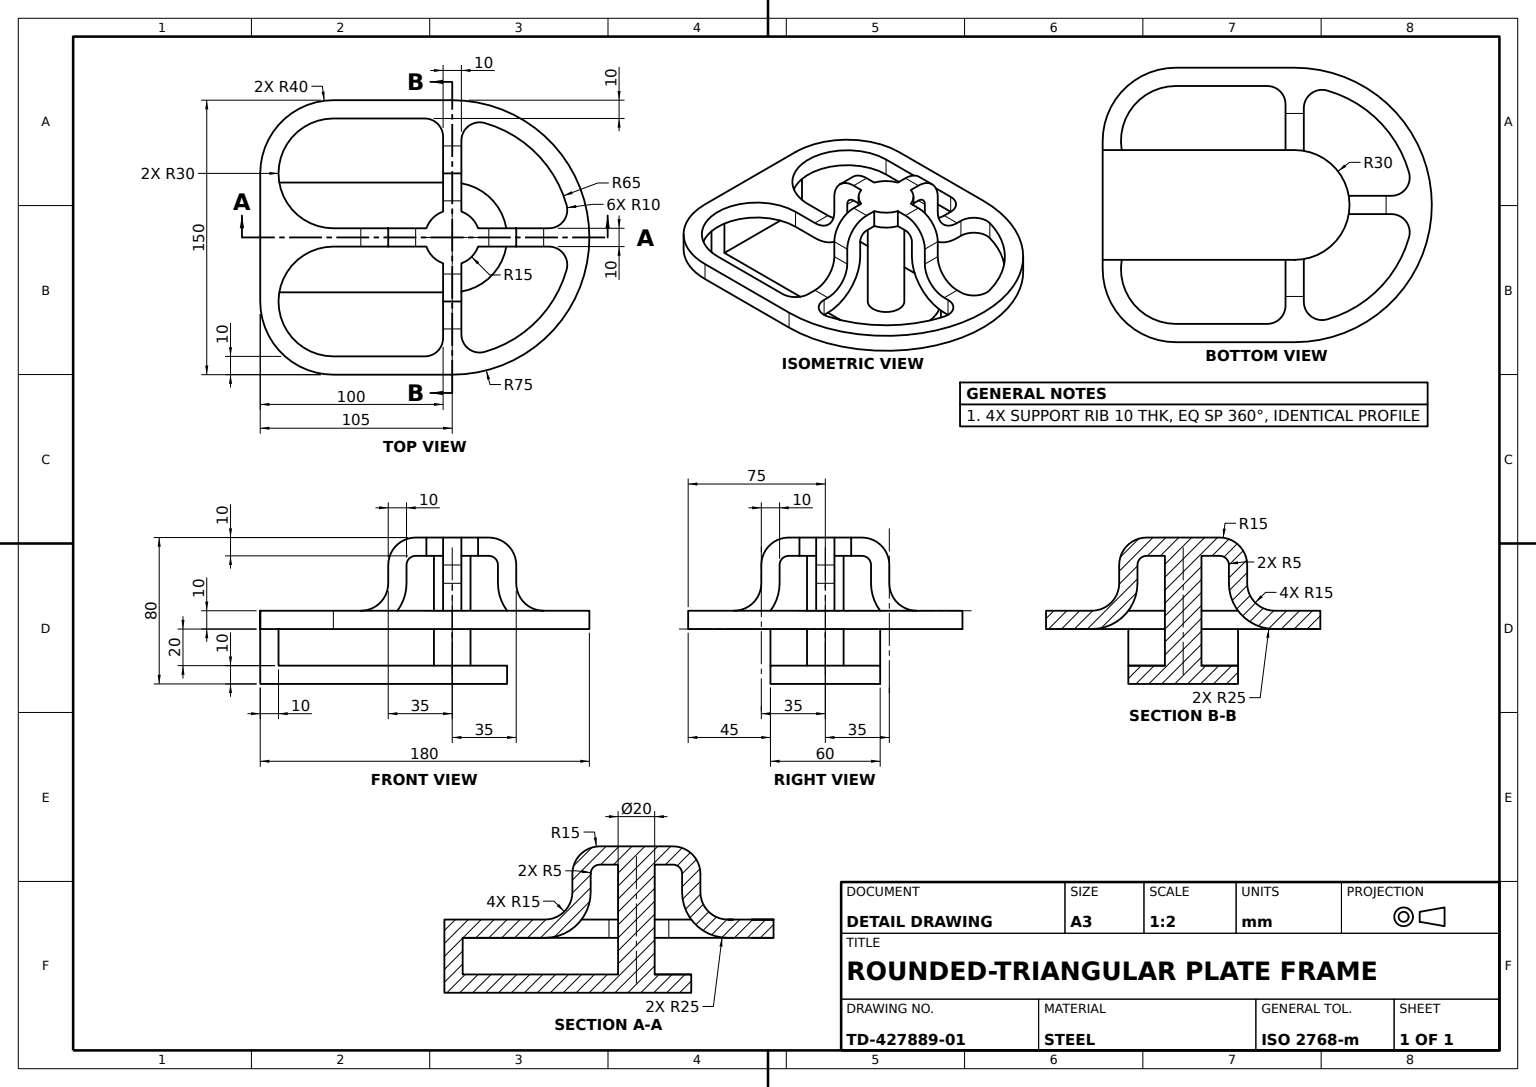
from build123d import *

# Parameters (mm, degrees)
CENTRAL_POST_SKETCH_R       = 10
CENTRAL_POST_20_DEPTH       = 40
MOUNTING_PLATE_DEPTH        = 10
RECTANGULAR_PAD_60X30_DEPTH = 10
SIDE_WALL_SKETCH_W          = 10
SIDE_WALL_SKETCH_H          = 20
SIDE_WALL_DEPTH             = 30
HUB_SKETCH_R                = 15
HUB_30_DEPTH                = 10
PLATE_CUTOUTS_SKETCH_R      = 10
PLATE_CUTOUTS_DEPTH         = 10
SUPPORT_RIB_DEPTH           = 5
RIB_PATTERN_4X_COUNT        = 4


with BuildPart() as part:
    # Central Post Sketch → Central Post Ø20 (new, symmetric)
    with BuildSketch(Plane(origin=(0, 0, 0), x_dir=(1, 0, 0), z_dir=(0, 1, 0))):
        with Locations(Location((0, 0, 0), (0, 0, 270))):
            Circle(CENTRAL_POST_SKETCH_R)
    extrude(amount=CENTRAL_POST_20_DEPTH, both=True)

    # Plate Outline Sketch → Mounting Plate (add)
    with BuildSketch(Plane(origin=(0, 0, 0), x_dir=(1, 0, 0), z_dir=(0, 1, 0))):
        with BuildLine():
            Line((-65, 75), (0, 75))
            ThreePointArc((0, 75), (75, 0), (0, -75))
            Line((0, -75), (-65, -75))
            ThreePointArc((-65, -75), (-93.284271247, -63.284271247), (-105, -35))
            Line((-105, -35), (-105, 35))
            ThreePointArc((-105, 35), (-93.284271247, 63.284271247), (-65, 75))
        make_face()
    extrude(amount=-MOUNTING_PLATE_DEPTH)

    # Pad Sketch → Rectangular Pad 60x30 (add)
    with BuildSketch(Plane.XZ.offset(40)):
        with BuildLine():
            Line((-105, 30), (0, 30))
            ThreePointArc((0, 30), (30, 0), (0, -30))
            Line((0, -30), (-105, -30))
            Line((-105, -30), (-105, 30))
        make_face()
    extrude(amount=-RECTANGULAR_PAD_60X30_DEPTH)

    # Side Wall Sketch → Side Wall (add, symmetric)
    with BuildSketch(Plane.XY):
        with Locations((-100, -20)):
            Rectangle(SIDE_WALL_SKETCH_W, SIDE_WALL_SKETCH_H)
    extrude(amount=SIDE_WALL_DEPTH, both=True)

    # Hub Sketch → Hub Ø30 (add)
    with BuildSketch(Plane(origin=(0, 40, 0), x_dir=(1, 0, 0), z_dir=(0, 1, 0))):
        with Locations(Location((0, 0, 0), (0, 0, 270))):
            Circle(HUB_SKETCH_R)
    extrude(amount=-HUB_30_DEPTH)

    # Plate Cutouts Sketch → Plate Cutouts (cut)
    with BuildSketch(Plane(origin=(0, 0, 0), x_dir=(1, 0, 0), z_dir=(0, 1, 0))):
        with BuildLine():
            ThreePointArc((62.53594008, 17.727272727), (45.961940777, 45.961940777), (17.727272727, 62.53594008))
            ThreePointArc((17.727272727, 62.53594008), (8.969773108, 60.892266573), (5, 52.915026221))
            Line((5, 52.915026221), (5, 50))
            Line((5, 50), (-5, 50))
            Line((-5, 50), (-5, 55))
            ThreePointArc((-5, 55), (-7.928932188, 62.071067812), (-15, 65))
            Line((-15, 65), (-65, 65))
            ThreePointArc((-65, 65), (-95, 35), (-65, 5))
            Line((-65, 5), (-65, -5))
            ThreePointArc((-65, -5), (-95, -35), (-65, -65))
            Line((-65, -65), (-15, -65))
            ThreePointArc((-15, -65), (-7.928932188, -62.071067812), (-5, -55))
            Line((-5, -55), (-5, -50))
            Line((-5, -50), (5, -50))
            Line((5, -50), (5, -52.915026221))
            ThreePointArc((5, -52.915026221), (8.969773108, -60.892266573), (17.727272727, -62.53594008))
            ThreePointArc((17.727272727, -62.53594008), (45.961940777, -45.961940777), (62.53594008, -17.727272727))
            ThreePointArc((62.53594008, -17.727272727), (60.892266573, -8.969773108), (52.915026221, -5))
            Line((52.915026221, -5), (52.915026221, 5))
            ThreePointArc((52.915026221, 5), (60.892266573, 8.969773108), (62.53594008, 17.727272727))
        make_face()
        with Locations(Location((0, 0, 0), (0, 0, 270))):
            Circle(PLATE_CUTOUTS_SKETCH_R, mode=Mode.SUBTRACT)
    extrude(amount=-PLATE_CUTOUTS_DEPTH, mode=Mode.SUBTRACT)

    # Support Rib Sketch → Support Rib (add, symmetric)
    with BuildSketch(Plane.XY):
        with BuildLine():
            Line((0, 40), (-20, 40))
            ThreePointArc((-20, 40), (-30.606601718, 35.606601718), (-35, 25))
            Line((-35, 25), (-35, 15))
            ThreePointArc((-35, 15), (-39.393398282, 4.393398282), (-50, 0))
            Line((-50, 0), (-65, 0))
            Line((-65, 0), (-65, -10))
            Line((-65, -10), (-50, -10))
            ThreePointArc((-50, -10), (-32.32233047, -2.67766953), (-25, 15))
            Line((-25, 15), (-25, 25))
            ThreePointArc((-25, 25), (-23.535533906, 28.535533906), (-20, 30))
            Line((-20, 30), (0, 30))
            Line((0, 30), (0, 40))
        make_face()
    support_rib = extrude(amount=SUPPORT_RIB_DEPTH, both=True)

    # Rib Pattern 4x: Support Rib ×4 about axis
    rib_pattern_4x_axis = Axis((0, 0, 0), (0, 1, 0))
    for i in range(1, RIB_PATTERN_4X_COUNT):
        add(support_rib.rotate(rib_pattern_4x_axis, i * 360 / RIB_PATTERN_4X_COUNT))


solid = part.part
